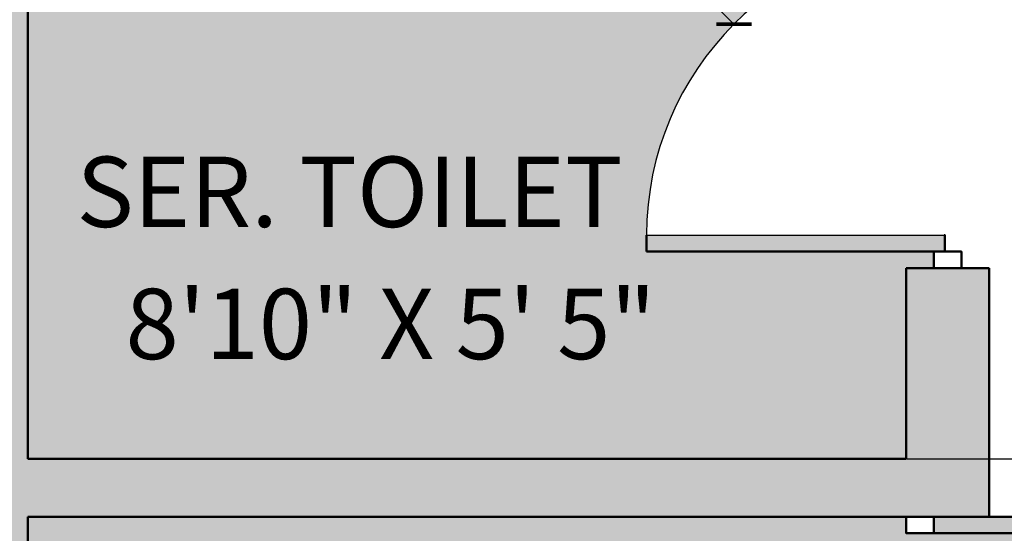
# Model space of a CAD drawing. Units: inches. Extents: x 925 to 2834, y 111 to 1355.
# Tile 10 of 25: x 1602 to 1721, y 820 to 882. Entities that reach past the tile are written whole.
import ezdxf

# ---------------------------------------------------------------- set-up
doc = ezdxf.new("R2010")
doc.units = ezdxf.units.IN
doc.header["$MEASUREMENT"] = 0
for name, color, linetype, lineweight in [('A-ANNO-DIMS', 2, 'Continuous', 18), ('A-AREA-IDEN', 7, 'Continuous', 18), ('A-DOOR', 2, 'Continuous', 25), ('A-FLOR-PATT', 252, 'Continuous', 13), ('A-WALL', 7, 'Continuous', 50)]:
    doc.layers.add(name, color=color, linetype=linetype, lineweight=lineweight)
doc.styles.get("Standard").update_dxf_attribs({"font": 'arial.ttf'})
doc.dimstyles.get("Standard").update_dxf_attribs({"dimtxt": 6, "dimasz": 3, "dimexe": 0.18, "dimexo": 0.0625, "dimgap": 0.09, "dimtad": 0, "dimtih": 1, "dimtoh": 1, "dimdec": 1, "dimzin": 0, "dimdsep": 46, "dimlunit": 3, "dimtxsty": 'Standard', "dimblk": 'ARCHTICK', "dimcen": 0.09, "dimadec": 0, "dimazin": 0, "dimtfac": 1, "dimtdec": 1, "dimtofl": 0, "dimtmove": 0, "dimatfit": 3, "dimfxl": 1, "dimtolj": 1, "dimtzin": 0, "dimarcsym": 0})

# ---------------------------------------------------------------- blocks, each defined once
blk = doc.blocks.new('_ArchTick')
at = {"color": 0, "linetype": 'ByBlock', "const_width": 0.15}
blk.add_lwpolyline([(-0.5, -0.5), (0.5, 0.5)], dxfattribs=at)
blk = doc.blocks.new('*D46')
at = {"layer": 'A-ANNO-DIMS', "color": 0, "lineweight": -2, "transparency": 16777216}
for p, q in [((1708.78, 828.59), (1988.62, 828.59)), ((1988.44, 828.59), (1988.44, 781.24)), ((1988.44, 727.59), (1988.44, 774.94)), ((1708.78, 727.59), (1988.62, 727.59))]:
    blk.add_line(p, q, dxfattribs=at)
at = {"layer": 'Defpoints', "color": 0, "transparency": 16777216}
for p in [(1708.71, 828.59), (1988.44, 828.59), (1708.71, 727.59)]:
    blk.add_point(p, dxfattribs=at)
at = {"layer": 'A-ANNO-DIMS', "color": 0, "lineweight": -2, "transparency": 16777216, "xscale": 3, "yscale": 3, "zscale": 3}
for p, rotation in [((1988.44, 828.59), 90), ((1988.44, 727.59), 270)]:
    blk.add_blockref('_ArchTick', p, dxfattribs=dict(at, rotation=rotation))
at = {"layer": 'A-ANNO-DIMS', "color": 0, "transparency": 16777216, "insert": (1988.44, 778.09), "char_height": 6, "attachment_point": 5}
blk.add_mtext('\\A1;101', dxfattribs=at)
blk = doc.blocks.new('*D47')
at = {"layer": 'A-ANNO-DIMS', "color": 0, "lineweight": -2, "transparency": 16777216}
for p, q in [((1708.78, 903.59), (1988.62, 903.59)), ((1988.44, 903.59), (1988.44, 869.23)), ((1988.44, 828.59), (1988.44, 862.95)), ((1708.78, 828.59), (1988.62, 828.59))]:
    blk.add_line(p, q, dxfattribs=at)
at = {"layer": 'Defpoints', "color": 0, "transparency": 16777216}
for p in [(1708.71, 903.59), (1988.44, 903.59), (1708.71, 828.59)]:
    blk.add_point(p, dxfattribs=at)
at = {"layer": 'A-ANNO-DIMS', "color": 0, "lineweight": -2, "transparency": 16777216, "xscale": 3, "yscale": 3, "zscale": 3}
for p, rotation in [((1988.44, 903.59), 90), ((1988.44, 828.59), 270)]:
    blk.add_blockref('_ArchTick', p, dxfattribs=dict(at, rotation=rotation))
at = {"layer": 'A-ANNO-DIMS', "color": 0, "transparency": 16777216, "insert": (1988.44, 866.09), "char_height": 6, "attachment_point": 5}
blk.add_mtext('\\A1;75', dxfattribs=at)
blk = doc.blocks.new('*D81')
at = {"layer": 'A-ANNO-DIMS', "color": 0, "lineweight": -2, "transparency": 16777216}
for p, q in [((1669.64, 896.32), (1672.64, 896.32)), ((1672.64, 896.32), (1687.92, 881.04)), ((1713.37, 855.5), (1713.37, 855.68)), ((1713.28, 855.59), (1713.46, 855.59))]:
    blk.add_line(p, q, dxfattribs=at)
at = {"layer": 'Defpoints', "color": 0, "transparency": 16777216}
for p in [(1687.92, 881.04), (1713.37, 855.59)]:
    blk.add_point(p, dxfattribs=at)
at = {"layer": 'A-ANNO-DIMS', "color": 0, "lineweight": -2, "transparency": 16777216, "xscale": 3, "yscale": 3, "zscale": 3, "rotation": 315.0000844046568}
blk.add_blockref('_ArchTick', (1687.92, 881.04), dxfattribs=at)
at = {"layer": 'A-ANNO-DIMS', "color": 0, "transparency": 16777216, "insert": (1655.94, 896.32), "char_height": 6, "attachment_point": 5}
blk.add_mtext('\\A1;3X R36', dxfattribs=at)

msp = doc.modelspace()

# ---------------------------------------------------------------- hatches: boundary and pattern name
at = {"layer": 'A-FLOR-PATT', "transparency": 33554605}
h = msp.add_hatch(color=256, dxfattribs=at)
h.dxf.hatch_style = 1
h.paths.add_polyline_path([(1931.688, 1294.5638), (991.7375, 1294.5638), (991.7375, 172.1134), (1931.688, 172.1134)])
h.paths.add_polyline_path([(1910.7128, 1273.5886), (1910.7128, 193.0886), (1012.7128, 193.0886), (1012.7128, 1273.5886)], flags=16)
h.paths.add_polyline_path([(1850.7128, 1213.5886), (1850.7128, 253.0886), (1072.7128, 253.0886), (1072.7128, 1213.5886)], flags=0)
h.paths.add_polyline_path([(1838.7128, 1201.5886), (1838.7128, 265.0886), (1084.7128, 265.0886), (1084.7128, 530.5886), (1084.7128, 1201.5886)], flags=0)
h.paths.add_polyline_path([(1547.6758, 1155.7396), (1547.6758, 1119.115), (1513.0687, 1119.115), (1513.0687, 1155.7396)], flags=0)
h.paths.add_polyline_path([(1600.1067, 1154.9439), (1634.7139, 1154.9439), (1634.7139, 1119.115), (1600.1067, 1119.115)], flags=0)
h.paths.add_polyline_path([(1505.2502, 1144.5358), (1505.2502, 1119.115), (1470.643, 1119.115), (1470.643, 1144.5358)], flags=0)
h.paths.add_polyline_path([(1559.1357, 1141.0962), (1593.7428, 1141.0962), (1593.7428, 1119.115), (1559.1357, 1119.115)], flags=0)
h.paths.add_polyline_path([(1462.8966, 1154.9439), (1462.8966, 1119.115), (1428.2895, 1119.115), (1428.2895, 1154.9439)], flags=0)
h.paths.add_polyline_path([(1642.4603, 1144.5358), (1677.0675, 1144.5358), (1677.0675, 1119.115), (1642.4603, 1119.115)], flags=0)
h.paths.add_polyline_path([(1422.3508, 1141.0962), (1422.3508, 1119.115), (1387.7436, 1119.115), (1387.7436, 1141.0962)], flags=0)
h.paths.add_polyline_path([(1684.8859, 1155.7396), (1719.4931, 1155.7396), (1719.4931, 1119.115), (1684.8859, 1119.115)], flags=0)
h.paths.add_polyline_path([(1718.7128, 1081.5886), (1718.7128, 1050.1249), (1715.7128, 1050.1249), (1715.7128, 1026.1249), (1715.7128, 1002.1249), (1718.7128, 1002.1249), (1730.7128, 1002.1249), (1730.7128, 998.1249), (1730.7128, 990.1249), (1730.7128, 986.1249), (1718.7128, 986.1249), (1718.7128, 893.5886), (1715.3735, 893.5886), (1715.3735, 891.5886), (1713.3735, 891.5886, 0.41421356), (1677.3735, 855.5886), (1713.3735, 855.5886), (1713.3735, 853.5886), (1715.3735, 853.5886), (1715.3735, 851.5886), (1718.7128, 851.5886), (1718.7128, 821.5865), (1734.4655, 821.5865), (1734.3735, 819.5886, -0.41421356), (1712.4415, 793.5886), (1712.4415, 791.5886), (1718.7128, 791.5886), (1718.7128, 717.5886), (1718.7128, 669.5886), (1732.7128, 669.5886), (1732.7128, 665.5886), (1732.7128, 641.5886), (1732.7128, 634.5886), (1732.7128, 610.5886), (1732.7128, 603.5886), (1718.7128, 603.5886), (1718.7128, 385.0886), (1434.2128, 385.0886), (1434.2128, 530.5886), (1410.2128, 530.5886), (1408.2128, 530.5886), (1408.2128, 532.5886, 0.41421356), (1372.2128, 568.5886), (1372.2128, 532.5886), (1370.2128, 532.5886), (1370.2128, 530.5886), (1368.2128, 530.5886), (1282.2128, 530.5886), (1210.2128, 530.5886), (1200.2128, 530.5886), (1200.2128, 542.1915), (1183.2307, 542.1915), (1183.2307, 546.1915), (1200.2128, 546.1915), (1200.2128, 572.1915), (1183.2307, 572.1915), (1183.2307, 576.1915), (1200.2128, 576.1915), (1200.2128, 727.5886), (1210.2128, 727.5886), (1234.2128, 727.5886), (1259.7128, 727.5886), (1259.7128, 775.5886), (1259.7128, 799.5886), (1259.7128, 847.5886), (1259.7128, 993.5872), (1259.7128, 1065.5872), (1259.7128, 1071.5886), (1219.6318, 1071.5886), (1219.6318, 1081.5886), (1084.7128, 1081.5886), (1084.7128, 1119.115), (1256.8974, 1119.115), (1256.8974, 1154.9439), (1291.5046, 1154.9439), (1291.5046, 1119.115), (1256.8974, 1119.115), (1256.6723, 1081.5886), (1293.7128, 1081.5886), (1341.7128, 1081.5886), (1341.7128, 1093.5886), (1347.7128, 1093.5886), (1371.7128, 1093.5886), (1377.7128, 1093.5886), (1377.7128, 1081.5886), (1668.7128, 1081.5886), (1668.7128, 1117.5886), (1675.7128, 1117.5886), (1711.7128, 1117.5886), (1718.7128, 1117.5886)], flags=0)
h.paths.add_polyline_path([(1376.2838, 1155.7396), (1376.2838, 1119.115), (1341.6766, 1119.115), (1341.6766, 1155.7396)], flags=0)
h.paths.add_polyline_path([(1341.7128, 1076.0886), (1293.7128, 1076.0886), (1293.7128, 1071.5886), (1269.7128, 1071.5886), (1269.7128, 1065.5872), (1266.7128, 1065.5872), (1266.7128, 1029.5872), (1265.7128, 1029.5872), (1265.7128, 993.5872), (1269.7128, 993.5872), (1269.7128, 903.5886), (1269.7128, 893.5886), (1269.7128, 847.5886), (1265.2128, 847.5886), (1265.2128, 799.5886), (1269.7128, 799.5886), (1269.7128, 775.5886), (1265.2128, 775.5886), (1265.2128, 727.5886), (1269.7128, 727.5886), (1444.2128, 727.5886), (1444.2128, 717.5886), (1234.2128, 717.5886), (1234.2128, 722.0886), (1210.2128, 722.0886), (1210.2128, 717.5886), (1210.2128, 540.5886), (1210.2128, 536.0886), (1282.2128, 536.0886), (1282.2128, 535.0886), (1210.2128, 535.0886), (1210.2128, 540.5886), (1210.2128, 717.5886), (1210.2128, 723.0886), (1234.2128, 723.0886), (1234.2128, 717.5886), (1444.2128, 717.5886), (1444.2128, 727.5886), (1269.7128, 727.5886), (1264.2128, 727.5886), (1264.2128, 775.5886), (1269.7128, 775.5886), (1269.7128, 799.5886), (1264.2128, 799.5886), (1264.2128, 847.5886), (1269.7128, 847.5886), (1269.7128, 893.5886), (1269.7128, 903.5886), (1269.7128, 993.5872), (1264.7128, 993.5872), (1264.7128, 1029.5872), (1265.7128, 1029.5872), (1265.7128, 1065.5872), (1269.7128, 1065.5872), (1269.7128, 1071.5886), (1293.7128, 1071.5886), (1293.7128, 1077.0886), (1341.7128, 1077.0886)], flags=0)
h.paths.add_polyline_path([(1730.9529, 1141.0962), (1765.5601, 1141.0962), (1765.5601, 1119.115), (1730.9529, 1119.115)], flags=0)
h.paths.add_polyline_path([(1333.8582, 1144.5358), (1333.8582, 1119.115), (1299.251, 1119.115), (1299.251, 1144.5358)], flags=0)
h.paths.add_polyline_path([(1592.7128, 968.5886), (1596.0342, 968.5886), (1602.7128, 968.5886), (1708.7128, 968.5886), (1708.7128, 903.5886), (1602.7128, 903.5886), (1602.7128, 938.5886), (1592.7128, 938.5886), (1592.7128, 903.5886), (1451.7128, 903.5886), (1451.7128, 893.5886), (1511.7128, 893.5886), (1511.7128, 881.5886), (1515.2128, 881.5886), (1518.7128, 881.5886), (1518.7128, 893.5886), (1592.7128, 893.5886), (1592.7128, 799.5886), (1518.7128, 799.5886), (1518.7128, 857.5886), (1511.7128, 857.5886), (1511.7128, 799.5886), (1511.7128, 772.0886), (1521.7128, 772.0886), (1521.7128, 792.5886), (1592.7128, 792.5886), (1592.7128, 727.5886), (1521.7128, 727.5886), (1521.7128, 748.0886), (1511.7128, 748.0886), (1511.7128, 717.5886), (1708.7128, 717.5886), (1714.2128, 717.5886), (1714.2128, 669.5886), (1708.7128, 669.5886), (1708.7128, 641.5886), (1492.2128, 641.5886), (1492.2128, 631.5886), (1621.2128, 631.5886), (1621.2128, 443.0886), (1625.7128, 443.0886), (1625.7128, 503.0886), (1625.7128, 507.5886), (1625.7128, 631.5886), (1708.7128, 631.5886), (1708.7128, 507.5886), (1655.7128, 507.5886), (1655.7128, 503.0886), (1708.7128, 503.0886), (1708.7128, 395.0886), (1625.7128, 395.0886), (1625.7128, 419.0886), (1621.2128, 419.0886), (1621.2128, 395.0886), (1482.2128, 395.0886), (1482.2128, 385.0886), (1434.2128, 385.0886), (1434.2128, 433.0886), (1444.2128, 433.0886), (1444.2128, 631.5886), (1450.2128, 631.5886), (1450.2128, 634.91), (1452.2128, 634.91), (1452.2128, 669.5886), (1454.2128, 669.5886, -0.40021217), (1490.1712, 635.3173), (1492.2128, 635.3173), (1492.2128, 641.5886), (1564.7128, 641.5886), (1564.7128, 677.5886), (1672.7128, 677.5886), (1672.7128, 681.5886), (1564.7128, 681.5886), (1564.7128, 717.5886), (1511.7128, 717.5886), (1511.7128, 748.0886), (1511.7128, 772.0886), (1511.7128, 799.5886), (1511.7128, 857.5886), (1511.8913, 857.5886), (1511.8913, 859.5886), (1515.6201, 859.5886, 0.41421356), (1537.552, 879.5886), (1513.552, 879.5886), (1511.8913, 879.5886), (1511.8913, 881.5886), (1511.7128, 881.5886), (1511.7128, 893.5886), (1451.7128, 893.5886), (1451.7128, 903.5886), (1592.7128, 903.5886), (1592.7128, 938.5886), (1592.7128, 940.5886), (1596.4415, 940.5886, 0.41421356), (1618.3735, 966.5886), (1594.3735, 966.5886), (1592.7128, 966.5886)], flags=0)
h.paths.add_polyline_path([(1377.7128, 903.5886), (1377.7128, 893.5886), (1305.7128, 893.5886), (1305.7128, 903.5886)], flags=0)
h.paths.add_polyline_path([(1708.7128, 821.5886), (1712.0342, 821.5886), (1712.0342, 819.5886), (1710.3735, 819.5886), (1708.7128, 819.5886)], flags=0)
h.paths.add_polyline_path([(1576.7128, 695.1992), (1575.5896, 693.6649), (1575.9687, 694.6994), (1575.4438, 695.1992), (1575.9687, 695.699), (1575.5896, 696.7335)], flags=0)
h.paths.add_polyline_path([(1565.9817, 662.3134), (1565.4568, 661.8136), (1565.8359, 660.7791), (1564.7128, 662.3134), (1565.8359, 663.8477), (1565.4568, 662.8132)], flags=0)
h.paths.add_polyline_path([(1444.2128, 433.0886), (1444.2128, 395.0886), (1482.2128, 395.0886), (1482.2128, 389.0886), (1438.2128, 389.0886), (1438.2128, 391.8608), (1438.2128, 433.0886)], flags=0)
h.paths.add_polyline_path([(1410.2128, 506.5886), (1410.2128, 289.0886), (1108.7128, 289.0886), (1108.7128, 506.5886)], flags=0)
h.paths.add_polyline_path([(1612.3153, 838.3016), (1680.4151, 838.3016), (1680.4151, 851.3131), (1612.3153, 851.3131)], flags=8)
h.paths.add_polyline_path([(1208.3174, 395.0436), (1282.1017, 395.0436), (1282.1017, 408.0552), (1208.3174, 408.0552)], flags=8)
h.paths.add_polyline_path([(1291.8049, 598.7427), (1369.8017, 598.7427), (1369.8017, 611.7542), (1291.8049, 611.7542)], flags=8)
h.paths.add_polyline_path([(1119.679, 917.3022), (1191.0817, 917.3022), (1191.0817, 930.3137), (1119.679, 930.3137)], flags=8)
h.paths.add_polyline_path([(1332.2261, 815.9808), (1410.2258, 815.9808), (1410.2258, 829.001), (1332.2261, 829.001)], flags=8)
h.paths.add_polyline_path([(1390.9013, 955.8158), (1475.4981, 955.8158), (1475.4981, 968.8273), (1390.9013, 968.8273)], flags=8)
h.paths.add_polyline_path([(1620.3436, 998.9325), (1688.4434, 998.9325), (1688.4434, 1011.944), (1620.3436, 1011.944)], flags=8)
h.paths.add_polyline_path([(1620.3436, 914.1039), (1691.7405, 914.1039), (1691.7405, 927.1155), (1620.3436, 927.1155)], flags=8)
h.paths.add_polyline_path([(1521.4542, 816.005), (1589.5569, 816.005), (1589.5569, 829.0253), (1521.4542, 829.0253)], flags=8)
h.paths.add_polyline_path([(1528.524, 740.3497), (1602.3082, 740.3497), (1602.3082, 753.3613), (1528.524, 753.3613)], flags=8)
h.paths.add_polyline_path([(1627.6094, 762.6128), (1702.3091, 762.6128), (1702.3091, 775.6244), (1627.6094, 775.6244)], flags=8)
h.paths.add_polyline_path([(1610.5442, 657.2751), (1684.3284, 657.2751), (1684.3284, 670.2867), (1610.5442, 670.2867)], flags=8)
h.paths.add_polyline_path([(1636.6983, 519.472), (1711.3981, 519.472), (1711.3981, 532.4835), (1636.6983, 532.4835)], flags=8)
h.paths.add_polyline_path([(1616.8577, 424.8539), (1694.8545, 424.8539), (1694.8545, 437.8654), (1616.8577, 437.8654)], flags=8)
h.paths.add_polyline_path([(1506.1456, 460.8838), (1579.9299, 460.8838), (1579.9299, 473.8953), (1506.1456, 473.8953)], flags=8)
h.paths.add_polyline_path([(1624.6119, 784.6011), (1696.9185, 784.6011), (1696.9185, 797.7864), (1624.6119, 797.7864)], flags=8)
h.paths.add_polyline_path([(1606.3732, 854.2194), (1683.3039, 854.2194), (1683.3039, 867.4048), (1606.3732, 867.4048)], flags=8)
h.paths.add_polyline_path([(1127.8008, 940.3581), (1165.1637, 940.3581), (1165.1637, 953.5348), (1127.8008, 953.5348)], flags=8)
h.paths.add_polyline_path([(1620.8657, 1019.4968), (1677.3447, 1019.4968), (1677.3447, 1032.6735), (1620.8657, 1032.6735)], flags=8)
h.paths.add_polyline_path([(1620.8643, 930.1821), (1703.0564, 930.1821), (1703.0564, 943.3675), (1620.8643, 943.3675)], flags=8)
h.paths.add_polyline_path([(1324.5702, 836.8338), (1408.0892, 836.8338), (1408.0892, 850.0191), (1324.5702, 850.0191)], flags=8)
h.paths.add_polyline_path([(1281.6584, 622.8885), (1383.6213, 622.8885), (1383.6213, 636.0739), (1281.6584, 636.0739)], flags=8)
h.paths.add_polyline_path([(1210.6721, 416.7893), (1269.1299, 416.7893), (1269.1299, 429.9747), (1210.6721, 429.9747)], flags=8)
h.paths.add_polyline_path([(1507.8264, 477.4836), (1586.7329, 477.4836), (1586.7329, 490.669), (1507.8264, 490.669)], flags=8)
h.paths.add_polyline_path([(1643.6238, 443.8135), (1696.6696, 443.8135), (1696.6696, 456.5643), (1643.6238, 456.5643)], flags=8)
h.paths.add_polyline_path([(1647.2466, 540.5638), (1693.1825, 540.5638), (1693.1825, 553.7491), (1647.2466, 553.7491)], flags=8)
h.paths.add_polyline_path([(1626.0633, 668.5064), (1673.3174, 668.5064), (1673.3174, 681.6831), (1626.0633, 681.6831)], flags=8)
h.paths.add_polyline_path([(1538.2915, 830.7872), (1567.5942, 830.7872), (1567.5942, 843.5293), (1538.2915, 843.5293)], flags=8)
h.paths.add_polyline_path([(1530.9338, 754.0477), (1559.576, 754.0477), (1559.576, 766.7898), (1530.9338, 766.7898)], flags=8)
h.paths.add_polyline_path([(1351.2461, 979.2309), (1513.8919, 979.2309), (1513.8919, 992.4076), (1351.2461, 992.4076)], flags=8)
at = {"layer": 'A-FLOR-PATT'}
h = msp.add_hatch(color=256, dxfattribs=at)
h.dxf.hatch_style = 1
h.paths.add_polyline_path([(1850.7128, 1213.5886), (1072.7128, 1213.5886), (1072.7128, 253.0886), (1850.7128, 253.0886)])
h.paths.add_polyline_path([(1084.7128, 1201.5886), (1838.7128, 1201.5886), (1838.7128, 265.0886), (1084.7128, 265.0886)], flags=16)
h.paths.add_polyline_path([(1183.2307, 576.1915), (1200.2128, 576.1915), (1200.2128, 727.5886), (1210.2128, 727.5886), (1234.2128, 727.5886), (1259.7128, 727.5886), (1259.7128, 775.5886), (1259.7128, 799.5886), (1259.7128, 847.5886), (1259.7128, 993.5872), (1259.7128, 1065.5872), (1259.7128, 1071.5886), (1219.6318, 1071.5886), (1219.6318, 1081.5886), (1293.7128, 1081.5886), (1341.7128, 1081.5886), (1341.7128, 1093.5886), (1347.7128, 1093.5886), (1347.7128, 1081.5886), (1371.7128, 1081.5886), (1371.7128, 1093.5886), (1377.7128, 1093.5886), (1377.7128, 1081.5886), (1668.7128, 1081.5886), (1668.7128, 1117.5886), (1675.7128, 1117.5886), (1675.7128, 1081.5886), (1711.7128, 1081.5886), (1711.7128, 1117.5886), (1718.7128, 1117.5886), (1718.7128, 1081.5886), (1718.7128, 1050.1249), (1715.7128, 1050.1249), (1715.7128, 1026.1249), (1715.7128, 1002.1249), (1718.7128, 1002.1249), (1730.7128, 1002.1249), (1730.7128, 998.1249), (1730.7128, 990.1249), (1730.7128, 986.1249), (1718.7128, 986.1249), (1718.7128, 893.5886), (1715.3735, 893.5886), (1715.3735, 891.5886), (1713.3735, 891.5886, 0.41421356), (1677.3735, 855.5886), (1713.3735, 855.5886), (1713.3735, 853.5886), (1715.3735, 853.5886), (1715.3735, 851.5886), (1718.7128, 851.5886), (1718.7128, 821.5865), (1734.4655, 821.5865), (1734.3735, 819.5886, -0.41421356), (1712.4415, 793.5886), (1712.4415, 791.5886), (1718.7128, 791.5886), (1718.7128, 717.5886), (1718.7128, 669.5886), (1732.7128, 669.5886), (1732.7128, 665.5886), (1732.7128, 641.5886), (1732.7128, 634.5886), (1732.7128, 610.5886), (1732.7128, 603.5886), (1718.7128, 603.5886), (1718.7128, 385.0886), (1434.2128, 385.0886), (1434.2128, 433.0886), (1434.2128, 530.5886), (1410.2128, 530.5886), (1408.2128, 530.5886), (1408.2128, 532.5886, 0.41421356), (1372.2128, 568.5886), (1372.2128, 532.5886), (1370.2128, 532.5886), (1370.2128, 530.5886), (1368.2128, 530.5886), (1282.2128, 530.5886), (1210.2128, 530.5886), (1200.2128, 530.5886), (1200.2128, 542.1915), (1183.2307, 542.1915), (1183.2307, 546.1915), (1200.2128, 546.1915), (1200.2128, 572.1915), (1183.2307, 572.1915)], flags=0)
h.paths.add_polyline_path([(1210.2128, 717.5886), (1210.2128, 723.0886), (1234.2128, 723.0886), (1234.2128, 717.5886), (1444.2128, 717.5886), (1444.2128, 727.5886), (1269.7128, 727.5886), (1264.2128, 727.5886), (1264.2128, 775.5886), (1269.7128, 775.5886), (1269.7128, 799.5886), (1264.2128, 799.5886), (1264.2128, 847.5886), (1269.7128, 847.5886), (1269.7128, 893.5886), (1269.7128, 903.5886), (1269.7128, 993.5872), (1264.7128, 993.5872), (1264.7128, 1029.5872), (1265.7128, 1029.5872), (1265.7128, 1065.5872), (1269.7128, 1065.5872), (1269.7128, 1071.5886), (1293.7128, 1071.5886), (1293.7128, 1077.0886), (1341.7128, 1077.0886), (1341.7128, 1076.0886), (1293.7128, 1076.0886), (1293.7128, 1071.5886), (1269.7128, 1071.5886), (1269.7128, 1065.5872), (1266.7128, 1065.5872), (1266.7128, 1029.5872), (1265.7128, 1029.5872), (1265.7128, 993.5872), (1269.7128, 993.5872), (1269.7128, 903.5886), (1269.7128, 893.5886), (1269.7128, 847.5886), (1265.2128, 847.5886), (1265.2128, 799.5886), (1269.7128, 799.5886), (1269.7128, 775.5886), (1265.2128, 775.5886), (1265.2128, 727.5886), (1269.7128, 727.5886), (1444.2128, 727.5886), (1444.2128, 717.5886), (1234.2128, 717.5886), (1234.2128, 722.0886), (1210.2128, 722.0886), (1210.2128, 717.5886), (1210.2128, 540.5886), (1210.2128, 536.0886), (1282.2128, 536.0886), (1282.2128, 535.0886), (1210.2128, 535.0886), (1210.2128, 540.5886)], flags=0)
h.paths.add_polyline_path([(1450.2128, 634.91), (1452.2128, 634.91), (1452.2128, 669.5886), (1454.2128, 669.5886, -0.40021217), (1490.1712, 635.3173), (1492.2128, 635.3173), (1492.2128, 641.5886), (1564.7128, 641.5886), (1564.7128, 677.5886), (1672.7128, 677.5886), (1672.7128, 681.5886), (1564.7128, 681.5886), (1564.7128, 717.5886), (1511.7128, 717.5886), (1511.7128, 748.0886), (1511.7128, 772.0886), (1511.7128, 799.5886), (1511.7128, 857.5886), (1511.8913, 857.5886), (1511.8913, 859.5886), (1515.6201, 859.5886, 0.41421356), (1537.552, 879.5886), (1513.552, 879.5886), (1511.8913, 879.5886), (1511.8913, 881.5886), (1511.7128, 881.5886), (1511.7128, 893.5886), (1451.7128, 893.5886), (1451.7128, 903.5886), (1592.7128, 903.5886), (1592.7128, 938.5886), (1592.7128, 940.5886), (1596.4415, 940.5886, 0.41421356), (1618.3735, 966.5886), (1594.3735, 966.5886), (1592.7128, 966.5886), (1592.7128, 968.5886), (1596.0342, 968.5886), (1602.7128, 968.5886), (1708.7128, 968.5886), (1708.7128, 903.5886), (1602.7128, 903.5886), (1602.7128, 938.5886), (1592.7128, 938.5886), (1592.7128, 903.5886), (1451.7128, 903.5886), (1451.7128, 893.5886), (1511.7128, 893.5886), (1511.7128, 881.5886), (1518.7128, 881.5886), (1518.7128, 893.5886), (1592.7128, 893.5886), (1592.7128, 799.5886), (1518.7128, 799.5886), (1518.7128, 857.5886), (1511.7128, 857.5886), (1511.7128, 799.5886), (1511.7128, 772.0886), (1521.7128, 772.0886), (1521.7128, 792.5886), (1592.7128, 792.5886), (1592.7128, 727.5886), (1521.7128, 727.5886), (1521.7128, 748.0886), (1511.7128, 748.0886), (1511.7128, 717.5886), (1708.7128, 717.5886), (1714.2128, 717.5886), (1714.2128, 669.5886), (1708.7128, 669.5886), (1708.7128, 641.5886), (1492.2128, 641.5886), (1492.2128, 631.5886), (1621.2128, 631.5886), (1621.2128, 443.0886), (1625.7128, 443.0886), (1625.7128, 503.0886), (1625.7128, 507.5886), (1625.7128, 631.5886), (1708.7128, 631.5886), (1708.7128, 507.5886), (1655.7128, 507.5886), (1655.7128, 503.0886), (1708.7128, 503.0886), (1708.7128, 395.0886), (1625.7128, 395.0886), (1625.7128, 419.0886), (1621.2128, 419.0886), (1621.2128, 395.0886), (1482.2128, 395.0886), (1482.2128, 389.0886), (1438.2128, 389.0886), (1438.2128, 391.8608), (1438.2128, 433.0886), (1444.2128, 433.0886), (1444.2128, 631.5886), (1450.2128, 631.5886)], flags=0)
h.paths.add_polyline_path([(1444.2128, 433.0886), (1444.2128, 395.0886), (1482.2128, 395.0886), (1482.2128, 391.0886), (1440.2128, 391.0886), (1440.2128, 391.8608), (1440.2128, 433.0886)], flags=0)
h.paths.add_polyline_path([(1305.7128, 893.5886), (1305.7128, 903.5886), (1377.7128, 903.5886), (1377.7128, 893.5886)], flags=0)
h.paths.add_polyline_path([(1564.7128, 662.3134), (1565.8359, 663.8477), (1565.4568, 662.8132), (1565.9817, 662.3134), (1565.4568, 661.8136), (1565.8359, 660.7791)], flags=0)
h.paths.add_polyline_path([(1575.4438, 695.1992), (1575.9687, 695.699), (1575.5896, 696.7335), (1576.7128, 695.1992), (1575.5896, 693.6649), (1575.9687, 694.6994)], flags=0)
h.paths.add_polyline_path([(1708.7128, 821.5886), (1712.0342, 821.5886), (1712.0342, 819.5886), (1710.3735, 819.5886), (1708.7128, 819.5886)], flags=0)
h = msp.add_hatch(color=256, dxfattribs=at)
h.dxf.hatch_style = 1
h.paths.add_polyline_path([(1718.7128, 603.5886), (1708.7128, 603.5886), (1708.7128, 507.5886), (1655.7128, 507.5886), (1655.7128, 503.0886), (1708.7128, 503.0886), (1708.7128, 395.0886), (1625.7128, 395.0886), (1625.7128, 419.0886), (1621.2128, 419.0886), (1621.2128, 395.0886), (1482.2128, 395.0886), (1482.2128, 385.0886), (1718.7128, 385.0886)])
h.paths.add_polyline_path([(1625.7128, 631.5886), (1708.7128, 631.5886), (1708.7128, 603.5886), (1718.7128, 603.5886), (1732.7128, 603.5886), (1732.7128, 610.5886), (1715.7128, 610.5886), (1715.7128, 634.5886), (1732.7128, 634.5886), (1732.7128, 641.5886), (1715.7128, 641.5886), (1715.7128, 665.5886), (1732.7128, 665.5886), (1732.7128, 669.5886), (1708.7128, 669.5886), (1708.7128, 641.5886), (1492.2128, 641.5886), (1492.2128, 631.5886), (1621.2128, 631.5886), (1621.2128, 443.0886), (1625.7128, 443.0886), (1625.7128, 503.0886), (1625.7128, 507.5886)])
h.paths.add_polyline_path([(1718.7128, 851.5886), (1708.7128, 851.5886), (1708.7128, 828.5886), (1602.7128, 828.5886), (1602.7128, 893.5886), (1708.7128, 893.5886), (1718.7128, 893.5886), (1718.7128, 986.1249), (1730.7128, 986.1249), (1730.7128, 990.1249), (1718.7128, 990.1249), (1718.7128, 998.1249), (1730.7128, 998.1249), (1730.7128, 1002.1249), (1718.7128, 1002.1249), (1708.7128, 1002.1249), (1708.7128, 975.5886), (1602.7128, 975.5886), (1602.7128, 1011.5886), (1592.7128, 1011.5886), (1592.7128, 968.5886), (1596.0342, 968.5886), (1602.7128, 968.5886), (1708.7128, 968.5886), (1708.7128, 903.5886), (1602.7128, 903.5886), (1602.7128, 938.5886), (1592.7128, 938.5886), (1592.7128, 903.5886), (1451.7128, 903.5886), (1451.7128, 893.5886), (1511.7128, 893.5886), (1511.7128, 881.5886), (1515.2128, 881.5886), (1518.7128, 881.5886), (1518.7128, 893.5886), (1592.7128, 893.5886), (1592.7128, 799.5886), (1518.7128, 799.5886), (1518.7128, 857.5886), (1511.7128, 857.5886), (1511.7128, 799.5886), (1511.7128, 772.0886), (1521.7128, 772.0886), (1521.7128, 792.5886), (1592.7128, 792.5886), (1592.7128, 727.5886), (1521.7128, 727.5886), (1521.7128, 748.0886), (1511.7128, 748.0886), (1511.7128, 717.5886), (1708.7128, 717.5886), (1718.7128, 717.5886), (1718.7128, 727.5886), (1718.7128, 791.5886), (1708.7128, 791.5886), (1708.7128, 727.5886), (1602.7128, 727.5886), (1602.7128, 821.5886), (1708.7128, 821.5886), (1712.0342, 821.5886), (1718.7128, 821.5886)])
h.paths.add_polyline_path([(1718.7128, 1081.5886), (1718.7128, 1117.5886), (1711.7128, 1117.5886), (1711.7128, 1081.5886), (1675.7128, 1081.5886), (1675.7128, 1117.5886), (1668.7128, 1117.5886), (1668.7128, 1081.5886), (1377.7128, 1081.5886), (1377.7128, 1093.5886), (1371.7128, 1093.5886), (1371.7128, 1081.5886), (1347.7128, 1081.5886), (1347.7128, 1093.5886), (1341.7128, 1093.5886), (1341.7128, 1081.5886), (1341.7128, 1071.5886), (1592.7128, 1071.5886), (1592.7128, 1035.5886), (1602.7128, 1035.5886), (1602.7128, 1071.5886), (1708.7128, 1071.5886), (1708.7128, 1050.1249), (1718.7128, 1050.1249)])
h.paths.add_polyline_path([(1293.7128, 1081.5886), (1219.6318, 1081.5886), (1219.6318, 1071.5886), (1259.7128, 1071.5886), (1259.7128, 1065.5872), (1269.7128, 1065.5872), (1269.7128, 1071.5886), (1293.7128, 1071.5886)])
h.paths.add_polyline_path([(1269.7128, 903.5886), (1269.7128, 993.5872), (1259.7128, 993.5872), (1259.7128, 847.5886), (1269.7128, 847.5886), (1269.7128, 893.5886)])
h.paths.add_polyline_path([(1377.7128, 903.5886), (1305.7128, 903.5886), (1305.7128, 893.5886), (1377.7128, 893.5886)])
h.paths.add_polyline_path([(1444.2128, 727.5886), (1269.7128, 727.5886), (1259.7128, 727.5886), (1234.2128, 727.5886), (1234.2128, 717.5886), (1444.2128, 717.5886)])
h.paths.add_polyline_path([(1269.7128, 799.5886), (1259.7128, 799.5886), (1259.7128, 775.5886), (1269.7128, 775.5886)])
h.paths.add_polyline_path([(1444.2128, 631.5886), (1450.2128, 631.5886), (1450.2128, 634.91), (1450.2128, 641.5886), (1434.2128, 641.5886), (1434.2128, 540.5886), (1410.2128, 540.5886), (1410.2128, 530.5886), (1434.2128, 530.5886), (1434.2128, 433.0886), (1444.2128, 433.0886)])
h.paths.add_polyline_path([(1368.2128, 533.91), (1368.2128, 540.5886), (1282.2128, 540.5886), (1282.2128, 530.5886), (1368.2128, 530.5886)])
h.paths.add_polyline_path([(1210.2128, 717.5886), (1210.2128, 727.5886), (1200.2128, 727.5886), (1200.2128, 576.1915), (1183.2307, 576.1915), (1183.2307, 572.1915), (1200.2128, 572.1915), (1200.2128, 546.1915), (1183.2307, 546.1915), (1183.2307, 542.1915), (1200.2128, 542.1915), (1200.2128, 530.5886), (1210.2128, 530.5886), (1210.2128, 540.5886)])
at = {"layer": 'A-FLOR-PATT', "transparency": 33554605}
h = msp.add_hatch(color=256, dxfattribs=at)
h.dxf.hatch_style = 1
h.paths.add_polyline_path([(1592.7128, 938.5886), (1592.7128, 940.5886), (1596.4415, 940.5886, 0.41421356), (1618.3735, 966.5886), (1594.3735, 966.5886), (1592.7128, 966.5886), (1592.7128, 968.5886), (1592.7128, 1011.5886), (1602.7128, 1011.5886), (1602.7128, 975.5886), (1708.7128, 975.5886), (1708.7128, 1002.1249), (1711.7128, 1002.1249), (1711.7128, 1026.1249), (1711.7128, 1050.1249), (1708.7128, 1050.1249), (1708.7128, 1071.5886), (1602.7128, 1071.5886), (1602.7128, 1035.5886), (1592.7128, 1035.5886), (1592.7128, 1071.5886), (1341.7128, 1071.5886), (1293.7128, 1071.5886), (1269.7128, 1071.5886), (1269.7128, 1065.5872), (1269.7128, 993.5872), (1269.7128, 903.5886), (1269.7128, 893.5886), (1269.7128, 847.5886), (1269.7128, 799.5886), (1269.7128, 775.5886), (1269.7128, 727.5886), (1444.2128, 727.5886), (1444.2128, 717.5886), (1234.2128, 717.5886), (1210.2128, 717.5886), (1210.2128, 540.5886), (1282.2128, 540.5886), (1368.2128, 540.5886), (1368.2128, 533.91), (1370.2128, 533.91), (1370.2128, 568.5886), (1372.2128, 568.5886, -0.40021217), (1408.1712, 534.3173), (1410.2128, 534.3173), (1410.2128, 540.5886), (1434.2128, 540.5886), (1434.2128, 641.5886), (1450.2128, 641.5886), (1450.2128, 634.91), (1452.2128, 634.91), (1452.2128, 669.5886), (1454.2128, 669.5886, -0.40021217), (1490.1712, 635.3173), (1492.2128, 635.3173), (1492.2128, 641.5886), (1564.7128, 641.5886), (1564.7128, 677.5886), (1672.7128, 677.5886), (1672.7128, 681.5886), (1564.7128, 681.5886), (1564.7128, 717.5886), (1511.7128, 717.5886), (1511.7128, 748.0886), (1511.7128, 772.0886), (1511.7128, 799.5886), (1511.7128, 857.5886), (1511.8913, 857.5886), (1511.8913, 859.5886), (1515.6201, 859.5886, 0.41421356), (1537.552, 879.5886), (1513.552, 879.5886), (1511.8913, 879.5886), (1511.8913, 881.5886), (1511.7128, 881.5886), (1511.7128, 893.5886), (1451.7128, 893.5886), (1451.7128, 903.5886), (1592.7128, 903.5886)])
h.paths.add_polyline_path([(1377.7128, 903.5886), (1377.7128, 893.5886), (1305.7128, 893.5886), (1305.7128, 903.5886)], flags=16)
h.paths.add_polyline_path([(1592.7128, 893.5886), (1518.7128, 893.5886), (1518.7128, 881.5865), (1537.6441, 881.5865), (1537.552, 879.5886, -0.41421356), (1515.6201, 859.5886), (1515.6201, 857.5886), (1518.7128, 857.5886), (1518.7128, 799.5886), (1592.7128, 799.5886)], flags=17)
h.paths.add_polyline_path([(1291.8049, 598.7427), (1369.8017, 598.7427), (1369.8017, 611.7542), (1291.8049, 611.7542)], flags=24)
h.paths.add_polyline_path([(1332.2261, 815.9808), (1410.2258, 815.9808), (1410.2258, 829.001), (1332.2261, 829.001)], flags=24)
h.paths.add_polyline_path([(1390.9013, 955.8158), (1475.4981, 955.8158), (1475.4981, 968.8273), (1390.9013, 968.8273)], flags=24)
h.paths.add_polyline_path([(1620.3436, 998.9325), (1688.4434, 998.9325), (1688.4434, 1011.944), (1620.3436, 1011.944)], flags=24)
h.paths.add_polyline_path([(1620.8657, 1019.4968), (1677.3447, 1019.4968), (1677.3447, 1032.6735), (1620.8657, 1032.6735)], flags=24)
h.paths.add_polyline_path([(1324.5702, 836.8338), (1408.0892, 836.8338), (1408.0892, 850.0191), (1324.5702, 850.0191)], flags=24)
h.paths.add_polyline_path([(1281.6584, 622.8885), (1383.6213, 622.8885), (1383.6213, 636.0739), (1281.6584, 636.0739)], flags=24)
h.paths.add_polyline_path([(1626.0633, 668.5064), (1673.3174, 668.5064), (1673.3174, 681.6831), (1626.0633, 681.6831)], flags=25)
h.paths.add_polyline_path([(1351.2461, 979.2309), (1513.8919, 979.2309), (1513.8919, 992.4076), (1351.2461, 992.4076)], flags=24)
h.paths.add_polyline_path([(1521.4542, 816.005), (1589.5569, 816.005), (1589.5569, 829.0253), (1521.4542, 829.0253)], flags=24)
h.paths.add_polyline_path([(1538.2915, 830.7872), (1567.5942, 830.7872), (1567.5942, 843.5293), (1538.2915, 843.5293)], flags=24)
h.paths.add_polyline_path([(1636.6983, 519.472), (1711.3981, 519.472), (1711.3981, 532.4835), (1636.6983, 532.4835)], flags=9)
h.paths.add_polyline_path([(1616.8577, 424.8539), (1694.8545, 424.8539), (1694.8545, 437.8654), (1616.8577, 437.8654)], flags=9)
h.paths.add_polyline_path([(1506.1456, 460.8838), (1579.9299, 460.8838), (1579.9299, 473.8953), (1506.1456, 473.8953)], flags=9)
h.paths.add_polyline_path([(1606.3732, 854.2194), (1683.3039, 854.2194), (1683.3039, 867.4048), (1606.3732, 867.4048)], flags=25)
h.paths.add_polyline_path([(1507.8264, 477.4836), (1586.7329, 477.4836), (1586.7329, 490.669), (1507.8264, 490.669)], flags=9)
h.paths.add_polyline_path([(1643.6238, 443.8135), (1696.6696, 443.8135), (1696.6696, 456.5643), (1643.6238, 456.5643)], flags=9)
h.paths.add_polyline_path([(1647.2466, 540.5638), (1693.1825, 540.5638), (1693.1825, 553.7491), (1647.2466, 553.7491)], flags=25)
h = msp.add_hatch(color=256, dxfattribs=at)
h.dxf.hatch_style = 1
h.paths.add_polyline_path([(1200.2128, 727.5886), (1084.7128, 727.5886), (1084.7128, 530.5886), (1200.2128, 530.5886), (1200.2128, 542.1915), (1183.2307, 542.1915), (1183.2307, 546.1915), (1200.2128, 546.1915), (1200.2128, 572.1915), (1183.2307, 572.1915), (1183.2307, 576.1915), (1200.2128, 576.1915)])
h.paths.add_polyline_path([(1612.3153, 838.3016), (1680.4151, 838.3016), (1680.4151, 851.3131), (1612.3153, 851.3131)], flags=9)
h.paths.add_polyline_path([(1291.8049, 598.7427), (1369.8017, 598.7427), (1369.8017, 611.7542), (1291.8049, 611.7542)], flags=9)
h.paths.add_polyline_path([(1119.679, 917.3022), (1191.0817, 917.3022), (1191.0817, 930.3137), (1119.679, 930.3137)], flags=9)
h.paths.add_polyline_path([(1332.2261, 815.9808), (1410.2258, 815.9808), (1410.2258, 829.001), (1332.2261, 829.001)], flags=9)
h.paths.add_polyline_path([(1390.9013, 955.8158), (1475.4981, 955.8158), (1475.4981, 968.8273), (1390.9013, 968.8273)], flags=9)
h.paths.add_polyline_path([(1620.3436, 998.9325), (1688.4434, 998.9325), (1688.4434, 1011.944), (1620.3436, 1011.944)], flags=9)
h.paths.add_polyline_path([(1620.3436, 914.1039), (1691.7405, 914.1039), (1691.7405, 927.1155), (1620.3436, 927.1155)], flags=9)
h.paths.add_polyline_path([(1521.4542, 816.005), (1589.5569, 816.005), (1589.5569, 829.0253), (1521.4542, 829.0253)], flags=9)
h.paths.add_polyline_path([(1522.4337, 740.3497), (1596.218, 740.3497), (1596.218, 753.3613), (1522.4337, 753.3613)], flags=9)
h.paths.add_polyline_path([(1606.3732, 854.2194), (1683.3039, 854.2194), (1683.3039, 867.4048), (1606.3732, 867.4048)], flags=9)
h.paths.add_polyline_path([(1127.8008, 940.3581), (1165.1637, 940.3581), (1165.1637, 953.5348), (1127.8008, 953.5348)], flags=9)
h.paths.add_polyline_path([(1620.8657, 1019.4968), (1677.3447, 1019.4968), (1677.3447, 1032.6735), (1620.8657, 1032.6735)], flags=9)
h.paths.add_polyline_path([(1620.8643, 930.1821), (1703.0564, 930.1821), (1703.0564, 943.3675), (1620.8643, 943.3675)], flags=9)
h.paths.add_polyline_path([(1324.5702, 836.8338), (1408.0892, 836.8338), (1408.0892, 850.0191), (1324.5702, 850.0191)], flags=9)
h.paths.add_polyline_path([(1281.6584, 622.8885), (1383.6213, 622.8885), (1383.6213, 636.0739), (1281.6584, 636.0739)], flags=9)
h.paths.add_polyline_path([(1626.0633, 668.5064), (1673.3174, 668.5064), (1673.3174, 681.6831), (1626.0633, 681.6831)], flags=9)
h.paths.add_polyline_path([(1538.2915, 830.7872), (1567.5942, 830.7872), (1567.5942, 843.5293), (1538.2915, 843.5293)], flags=9)
h.paths.add_polyline_path([(1351.2461, 979.2309), (1513.8919, 979.2309), (1513.8919, 992.4076), (1351.2461, 992.4076)], flags=9)
h = msp.add_hatch(color=256, dxfattribs=at)
h.dxf.hatch_style = 1
h.paths.add_polyline_path([(1621.2128, 631.5886), (1492.2128, 631.5886), (1490.2128, 631.5886), (1490.2128, 633.5886, 0.41421356), (1454.2128, 669.5886), (1454.2128, 633.5886), (1452.2128, 633.5886), (1452.2128, 631.5886), (1450.2128, 631.5886), (1444.2128, 631.5886), (1444.2128, 395.0886), (1482.2128, 395.0886), (1621.2128, 395.0886), (1621.2128, 419.0886), (1625.7128, 419.0886), (1625.7128, 395.0886), (1708.7128, 395.0886), (1708.7128, 503.0886), (1655.7128, 503.0886), (1655.7128, 507.5886), (1708.7128, 507.5886), (1708.7128, 631.5886), (1625.7128, 631.5886), (1625.7128, 507.5886), (1625.7128, 503.0886), (1625.7128, 443.0886), (1621.2128, 443.0886)])
h.paths.add_polyline_path([(1636.6983, 519.472), (1711.3981, 519.472), (1711.3981, 532.4835), (1636.6983, 532.4835)], flags=9)
h.paths.add_polyline_path([(1616.8577, 424.8539), (1694.8545, 424.8539), (1694.8545, 437.8654), (1616.8577, 437.8654)], flags=24)
h.paths.add_polyline_path([(1506.1456, 460.8838), (1579.9299, 460.8838), (1579.9299, 473.8953), (1506.1456, 473.8953)], flags=24)
h.paths.add_polyline_path([(1507.8264, 477.4836), (1586.7329, 477.4836), (1586.7329, 490.669), (1507.8264, 490.669)], flags=24)
h.paths.add_polyline_path([(1643.6238, 443.8135), (1696.6696, 443.8135), (1696.6696, 456.5643), (1643.6238, 456.5643)], flags=24)
h.paths.add_polyline_path([(1647.2466, 540.5638), (1693.1825, 540.5638), (1693.1825, 553.7491), (1647.2466, 553.7491)], flags=24)
h.paths.add_polyline_path([(1612.3153, 838.3016), (1680.4151, 838.3016), (1680.4151, 851.3131), (1612.3153, 851.3131)], flags=9)
h.paths.add_polyline_path([(1291.8049, 598.7427), (1369.8017, 598.7427), (1369.8017, 611.7542), (1291.8049, 611.7542)], flags=9)
h.paths.add_polyline_path([(1119.679, 917.3022), (1191.0817, 917.3022), (1191.0817, 930.3137), (1119.679, 930.3137)], flags=9)
h.paths.add_polyline_path([(1332.2261, 815.9808), (1410.2258, 815.9808), (1410.2258, 829.001), (1332.2261, 829.001)], flags=9)
h.paths.add_polyline_path([(1390.9013, 955.8158), (1475.4981, 955.8158), (1475.4981, 968.8273), (1390.9013, 968.8273)], flags=9)
h.paths.add_polyline_path([(1620.3436, 998.9325), (1688.4434, 998.9325), (1688.4434, 1011.944), (1620.3436, 1011.944)], flags=9)
h.paths.add_polyline_path([(1620.3436, 914.1039), (1691.7405, 914.1039), (1691.7405, 927.1155), (1620.3436, 927.1155)], flags=9)
h.paths.add_polyline_path([(1521.4542, 816.005), (1589.5569, 816.005), (1589.5569, 829.0253), (1521.4542, 829.0253)], flags=9)
h.paths.add_polyline_path([(1528.524, 740.3497), (1602.3082, 740.3497), (1602.3082, 753.3613), (1528.524, 753.3613)], flags=9)
h.paths.add_polyline_path([(1627.6094, 762.6128), (1702.3091, 762.6128), (1702.3091, 775.6244), (1627.6094, 775.6244)], flags=9)
h.paths.add_polyline_path([(1624.6119, 784.6011), (1696.9185, 784.6011), (1696.9185, 797.7864), (1624.6119, 797.7864)], flags=9)
h.paths.add_polyline_path([(1606.3732, 854.2194), (1683.3039, 854.2194), (1683.3039, 867.4048), (1606.3732, 867.4048)], flags=9)
h.paths.add_polyline_path([(1127.8008, 940.3581), (1165.1637, 940.3581), (1165.1637, 953.5348), (1127.8008, 953.5348)], flags=9)
h.paths.add_polyline_path([(1620.8657, 1019.4968), (1677.3447, 1019.4968), (1677.3447, 1032.6735), (1620.8657, 1032.6735)], flags=9)
h.paths.add_polyline_path([(1620.8643, 930.1821), (1703.0564, 930.1821), (1703.0564, 943.3675), (1620.8643, 943.3675)], flags=9)
h.paths.add_polyline_path([(1324.5702, 836.8338), (1408.0892, 836.8338), (1408.0892, 850.0191), (1324.5702, 850.0191)], flags=9)
h.paths.add_polyline_path([(1281.6584, 622.8885), (1383.6213, 622.8885), (1383.6213, 636.0739), (1281.6584, 636.0739)], flags=9)
h.paths.add_polyline_path([(1626.0633, 668.5064), (1673.3174, 668.5064), (1673.3174, 681.6831), (1626.0633, 681.6831)], flags=9)
h.paths.add_polyline_path([(1538.2915, 830.7872), (1567.5942, 830.7872), (1567.5942, 843.5293), (1538.2915, 843.5293)], flags=9)
h.paths.add_polyline_path([(1530.9338, 754.0477), (1559.576, 754.0477), (1559.576, 766.7898), (1530.9338, 766.7898)], flags=9)
h.paths.add_polyline_path([(1351.2461, 979.2309), (1513.8919, 979.2309), (1513.8919, 992.4076), (1351.2461, 992.4076)], flags=9)
h = msp.add_hatch(color=256, dxfattribs=at)
h.dxf.hatch_style = 1
h.paths.add_polyline_path([(1708.7128, 791.5886), (1708.7128, 793.5886), (1712.4415, 793.5886, 0.41421356), (1734.3735, 819.5886), (1710.3735, 819.5886), (1708.7128, 819.5886), (1708.7128, 821.5886), (1602.7128, 821.5886), (1602.7128, 727.5886), (1708.7128, 727.5886)])
h.paths.add_polyline_path([(1708.7128, 851.5886), (1712.052, 851.5886), (1712.052, 853.5886), (1677.3735, 853.5886), (1677.3735, 855.5886, -0.40021217), (1711.6447, 891.5471), (1711.6447, 893.5886), (1708.7128, 893.5886), (1602.7128, 893.5886), (1602.7128, 828.5886), (1708.7128, 828.5886)])
h.paths.add_polyline_path([(1708.7128, 968.5886), (1618.4656, 968.5886), (1618.3735, 966.5886, -0.41421356), (1596.4415, 940.5886), (1596.4415, 938.5886), (1602.7128, 938.5886), (1602.7128, 903.5886), (1708.7128, 903.5886)])
h.paths.add_polyline_path([(1708.7128, 717.5886), (1672.7128, 717.5886), (1672.7128, 641.5886), (1708.7128, 641.5886)])
h.paths.add_polyline_path([(1588.7128, 717.5886), (1576.7128, 717.5886), (1576.7128, 681.5886), (1588.7128, 681.5886)])
h.paths.add_polyline_path([(1576.7128, 717.5886), (1564.7128, 717.5886), (1564.7128, 695.1992), (1575.4438, 695.1992), (1575.9687, 695.699), (1575.5896, 696.7335), (1576.7128, 695.1992)])
h.paths.add_polyline_path([(1576.7128, 695.1992), (1575.5896, 693.6649), (1575.9687, 694.6994), (1575.4438, 695.1992), (1564.7128, 695.1992), (1564.7128, 681.5886), (1576.7128, 681.5886)])
h.paths.add_polyline_path([(1600.7128, 717.5886), (1588.7128, 717.5886), (1588.7128, 681.5886), (1600.7128, 681.5886)])
h.paths.add_polyline_path([(1612.7128, 717.5886), (1600.7128, 717.5886), (1600.7128, 681.5886), (1612.7128, 681.5886)])
h.paths.add_polyline_path([(1624.7128, 717.5886), (1612.7128, 717.5886), (1612.7128, 681.5886), (1624.7128, 681.5886)])
h.paths.add_polyline_path([(1636.7128, 717.5886), (1624.7128, 717.5886), (1624.7128, 681.5886), (1636.7128, 681.5886)])
h.paths.add_polyline_path([(1648.7128, 717.5886), (1636.7128, 717.5886), (1636.7128, 681.5886), (1648.7128, 681.5886)])
h.paths.add_polyline_path([(1660.7128, 717.5886), (1648.7128, 717.5886), (1648.7128, 681.5886), (1660.7128, 681.5886)])
h.paths.add_polyline_path([(1672.7128, 717.5886), (1660.7128, 717.5886), (1660.7128, 681.5886), (1672.7128, 681.5886)])
h.paths.add_polyline_path([(1576.7128, 662.3134), (1565.9817, 662.3134), (1565.4568, 661.8136), (1565.8359, 660.7791), (1564.7128, 662.3134), (1564.7128, 641.5886), (1576.7128, 641.5886)])
h.paths.add_polyline_path([(1576.7128, 677.5886), (1564.7128, 677.5886), (1564.7128, 662.3134), (1565.8359, 663.8477), (1565.4568, 662.8132), (1565.9817, 662.3134), (1576.7128, 662.3134)])
h.paths.add_polyline_path([(1588.7128, 677.5886), (1576.7128, 677.5886), (1576.7128, 641.5886), (1588.7128, 641.5886)])
h.paths.add_polyline_path([(1600.7128, 677.5886), (1588.7128, 677.5886), (1588.7128, 641.5886), (1600.7128, 641.5886)])
h.paths.add_polyline_path([(1612.7128, 677.5886), (1600.7128, 677.5886), (1600.7128, 641.5886), (1612.7128, 641.5886)])
h.paths.add_polyline_path([(1624.7128, 677.5886), (1612.7128, 677.5886), (1612.7128, 641.5886), (1624.7128, 641.5886)])
h.paths.add_polyline_path([(1636.7128, 677.5886), (1624.7128, 677.5886), (1624.7128, 641.5886), (1636.7128, 641.5886)])
h.paths.add_polyline_path([(1648.7128, 677.5886), (1636.7128, 677.5886), (1636.7128, 641.5886), (1648.7128, 641.5886)])
h.paths.add_polyline_path([(1660.7128, 677.5886), (1648.7128, 677.5886), (1648.7128, 641.5886), (1660.7128, 641.5886)])
h.paths.add_polyline_path([(1672.7128, 677.5886), (1660.7128, 677.5886), (1660.7128, 641.5886), (1672.7128, 641.5886)])
h.paths.add_polyline_path([(1627.6094, 762.6128), (1702.3091, 762.6128), (1702.3091, 775.6244), (1627.6094, 775.6244)], flags=24)
h.paths.add_polyline_path([(1624.6119, 784.6011), (1696.9185, 784.6011), (1696.9185, 797.7864), (1624.6119, 797.7864)], flags=24)
h.paths.add_polyline_path([(1612.3153, 838.3016), (1680.4151, 838.3016), (1680.4151, 851.3131), (1612.3153, 851.3131)], flags=24)
h.paths.add_polyline_path([(1606.3732, 854.2194), (1683.3039, 854.2194), (1683.3039, 867.4048), (1606.3732, 867.4048)], flags=24)
h.paths.add_polyline_path([(1620.3436, 914.1039), (1691.7405, 914.1039), (1691.7405, 927.1155), (1620.3436, 927.1155)], flags=24)
h.paths.add_polyline_path([(1620.8643, 930.1821), (1703.0564, 930.1821), (1703.0564, 943.3675), (1620.8643, 943.3675)], flags=24)
h.paths.add_polyline_path([(1610.5442, 657.2751), (1684.3284, 657.2751), (1684.3284, 670.2867), (1610.5442, 670.2867)], flags=9)
h.paths.add_polyline_path([(1626.0633, 668.5064), (1673.3174, 668.5064), (1673.3174, 681.6831), (1626.0633, 681.6831)], flags=9)
at = {"layer": 'A-FLOR-PATT'}
h = msp.add_hatch(color=256, dxfattribs=at)
h.dxf.hatch_style = 1
h.paths.add_polyline_path([(1713.3735, 855.5886), (1677.3735, 855.5886), (1677.3735, 853.5886), (1713.3735, 853.5886)])
h.paths.add_polyline_path([(1372.2128, 568.5886), (1370.2128, 568.5886), (1370.2128, 532.5886), (1372.2128, 532.5886)])
h.paths.add_polyline_path([(1734.4655, 821.5865), (1712.0342, 821.5865), (1712.0342, 819.5886), (1734.3735, 819.5886)])
h.paths.add_polyline_path([(1454.2128, 669.5886), (1452.2128, 669.5886), (1452.2128, 633.5886), (1454.2128, 633.5886)])
h.paths.add_polyline_path([(1537.6441, 881.5865), (1515.2128, 881.5865), (1515.2128, 879.5886), (1537.552, 879.5886)])

# ---------------------------------------------------------------- linework, layer by layer
at = {"layer": 'A-DOOR'}
msp.add_line((1677.3735, 855.5886), (1713.3735, 855.5886), dxfattribs=at)
msp.add_arc((1713.3735, 855.5886), 36, 90, 180, dxfattribs=at)
at = {"layer": 'A-WALL'}
for p, q in [((1602.7128, 893.5886), (1602.7128, 828.5886)), ((1677.3735, 853.5886), (1677.3735, 855.5886)), ((1713.3735, 855.5886), (1713.3735, 853.5886)), ((1713.3735, 855.5886), (1713.3735, 853.5886)), ((1713.3735, 853.5886), (1677.3735, 853.5886)), ((1713.3735, 853.5886), (1715.3735, 853.5886)), ((1715.3735, 853.5886), (1715.3735, 851.5886)), ((1708.7128, 851.5886), (1708.7128, 828.5886)), ((1708.7128, 851.5886), (1718.7128, 851.5886)), ((1715.3735, 851.5886), (1718.7128, 851.5886)), ((1718.7128, 851.5886), (1718.7128, 821.5886)), ((1718.7128, 851.5886), (1718.7128, 821.5886)), ((1602.7128, 828.5886), (1708.7128, 828.5886)), ((1602.7128, 821.5886), (1708.7128, 821.5886)), ((1602.7128, 821.5886), (1602.7128, 727.5886)), ((1708.7128, 821.5886), (1718.7128, 821.5886)), ((1734.4655, 821.5865), (1712.0342, 821.5865)), ((1718.7128, 821.5886), (1734.4655, 821.5865)), ((1710.3735, 819.5886), (1734.3735, 819.5886))]:
    msp.add_line(p, q, dxfattribs=at)
for points in [[(1712.052, 851.5886), (1712.052, 853.5886), (1715.3735, 853.5886), (1715.3735, 851.5886)], [(1712.0342, 821.5886), (1712.0342, 819.5886), (1708.7128, 819.5886), (1708.7128, 821.5886)]]:
    msp.add_lwpolyline(points, close=True, dxfattribs=at)

# ---------------------------------------------------------------- texts
at = {"layer": 'A-AREA-IDEN'}
for s, p in [('SER. TOILET', (1608.5708, 856.5619)), ('8\'10" X 5\' 5"', (1614.4838, 840.615))]:
    msp.add_text(s, height=8.494735, dxfattribs=at).set_placement(p)

# ---------------------------------------------------------------- dimensions: what is measured, and where the dimension line sits
at = {"layer": 'A-ANNO-DIMS'}
dim = msp.add_radius_dim(center=(1713.3735, 855.5886), mpoint=(1687.9176, 881.0444), text='3X <>', dimstyle='Standard', override={"dimdec": 0, "dimlfac": 1, "dimrnd": 0, "dimzin": 0, "dimdsep": 46, "dimlunit": 2}, dxfattribs=at)
dim.commit()
dim.dimension.update_dxf_attribs({"geometry": '*D81', "text_midpoint": (1655.9436, 896.3179), "dimtype": 164})
for base, p1, p2, picture, middle in [((1988.438, 903.5886), (1708.7128, 828.5886), (1708.7128, 903.5886), '*D47', (1988.438, 866.0886)), ((1988.438, 828.5886), (1708.7128, 727.5886), (1708.7128, 828.5886), '*D46', (1988.438, 778.0886))]:
    dim = msp.add_linear_dim(base=base, p1=p1, p2=p2, angle=90, dimstyle='Standard', override={"dimdec": 0, "dimlfac": 1, "dimrnd": 0, "dimzin": 0, "dimdsep": 46, "dimlunit": 2}, dxfattribs=at)
    dim.commit()
    dim.dimension.update_dxf_attribs({"geometry": picture, "text_midpoint": middle})

doc.saveas('drawing.dxf')
